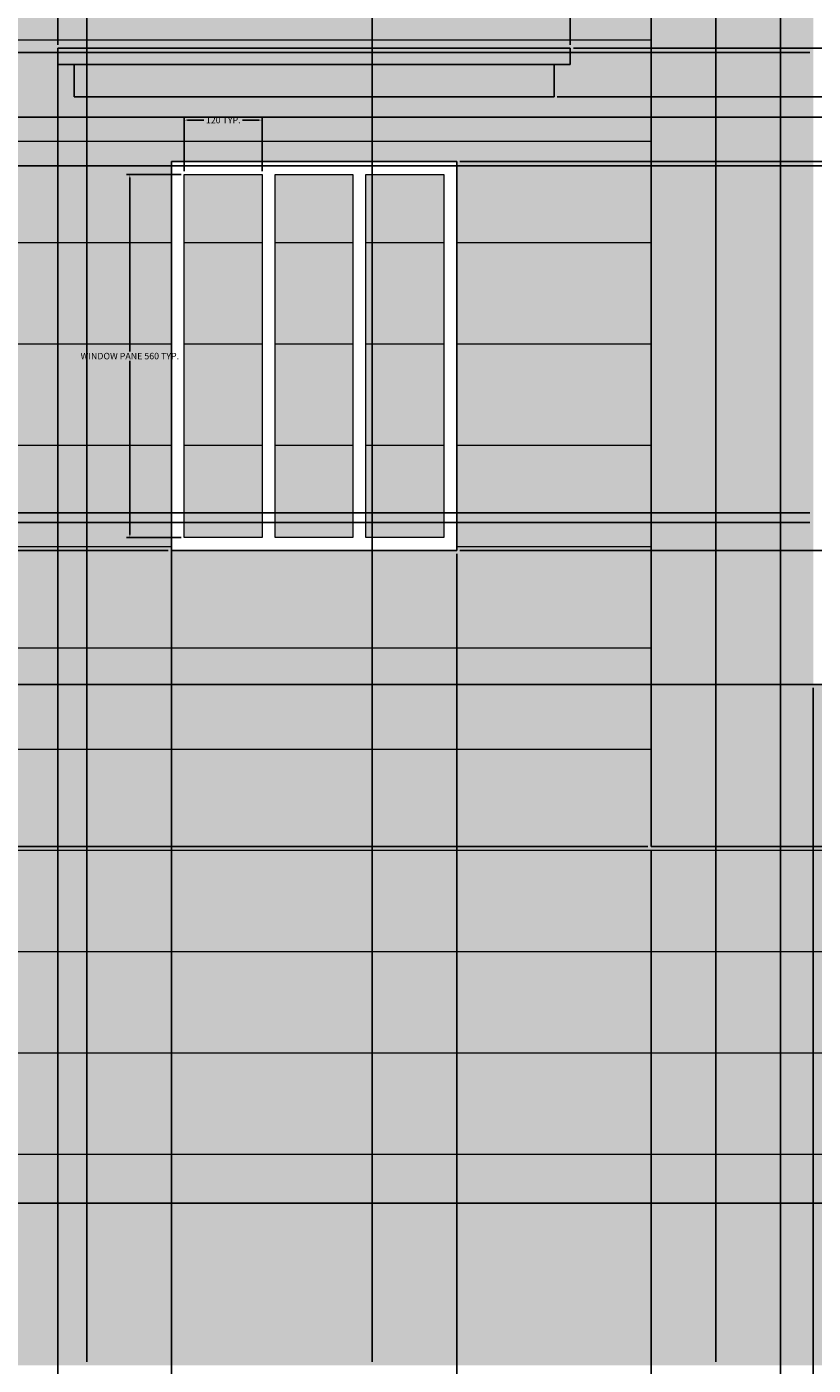
# Model space of a CAD drawing. Units: millimetres. Extents: x 2970 to 7764, y 2196 to 7505.
# Tile 9 of 13: x 4793 to 6006, y 4206 to 6270. Entities that reach past the tile are written whole.
import ezdxf

# ---------------------------------------------------------------- set-up
doc = ezdxf.new("R2010")
doc.units = ezdxf.units.MM
doc.header["$MEASUREMENT"] = 0
for name, color, linetype, lineweight in [('A-ANNO-DIMS', 2, 'Continuous', 18), ('A-ELEV', 7, 'Continuous', 25), ('A-ELEV-PATT', 8, 'Continuous', 13), ('A-GLAZ', 4, 'Continuous', 18)]:
    doc.layers.add(name, color=color, linetype=linetype, lineweight=lineweight)
doc.styles.get("Standard").update_dxf_attribs({"font": 'arial.ttf'})
doc.dimstyles.get("Standard").update_dxf_attribs({"dimtxt": 10, "dimasz": 5, "dimexe": 5, "dimexo": 5, "dimgap": 2, "dimtad": 0, "dimtih": 1, "dimtoh": 1, "dimdec": 0, "dimzin": 0, "dimdsep": 46, "dimtxsty": 'Standard', "dimcen": 2, "dimadec": 0, "dimazin": 0, "dimtfac": 1, "dimtdec": 0, "dimtofl": 0, "dimtmove": 0, "dimatfit": 3, "dimfxl": 1, "dimtolj": 1, "dimtzin": 0, "dimarcsym": 0})

# ---------------------------------------------------------------- blocks, each defined once
blk = doc.blocks.new('WIN-PANE')
blk.add_line((120, 560), (120, 0))
blk.add_lwpolyline([(120, 0), (0, 0), (0, 560), (120, 560)])
blk = doc.blocks.new('*D4')
at = {"layer": 'A-ANNO-DIMS', "color": 0, "lineweight": -2, "transparency": 16777216}
for p, q in [((5030.8, 6042.5), (4946.8, 6042.5)), ((4951.8, 6037.5), (4951.8, 5769.7)), ((4951.8, 5487.5), (4951.8, 5755.3)), ((5030.8, 5482.5), (4946.8, 5482.5))]:
    blk.add_line(p, q, dxfattribs=at)
at = {"layer": 'A-ANNO-DIMS', "color": 0, "transparency": 16777216}
for points in [[(4951, 6037.5), (4952.6, 6037.5), (4951.8, 6042.5)], [(4951, 5487.5), (4952.6, 5487.5), (4951.8, 5482.5)]]:
    blk.add_solid(points, dxfattribs=at)
at = {"layer": 'Defpoints', "color": 0, "transparency": 16777216}
for p in [(4951.8, 6042.5), (5035.8, 6042.5), (5035.8, 5482.5)]:
    blk.add_point(p, dxfattribs=at)
at = {"layer": 'A-ANNO-DIMS', "color": 0, "transparency": 16777216, "insert": (4951.8, 5762.5), "char_height": 10, "attachment_point": 5}
blk.add_mtext('\\A1;WINDOW PANE 560 TYP.', dxfattribs=at)
blk = doc.blocks.new('*D5')
at = {"layer": 'A-ANNO-DIMS', "color": 0, "lineweight": -2, "transparency": 16777216}
for p, q in [((5035.8, 6047.5), (5035.8, 6131.5)), ((5040.8, 6126.5), (5066.1, 6126.5)), ((5150.8, 6126.5), (5125.6, 6126.5)), ((5155.8, 6047.5), (5155.8, 6131.5))]:
    blk.add_line(p, q, dxfattribs=at)
at = {"layer": 'A-ANNO-DIMS', "color": 0, "transparency": 16777216}
for points in [[(5040.8, 6127.3), (5040.8, 6125.7), (5035.8, 6126.5)], [(5150.8, 6127.3), (5150.8, 6125.7), (5155.8, 6126.5)]]:
    blk.add_solid(points, dxfattribs=at)
at = {"layer": 'Defpoints', "color": 0, "transparency": 16777216}
for p in [(5155.8, 6126.5), (5035.8, 6042.5), (5155.8, 6042.5)]:
    blk.add_point(p, dxfattribs=at)
at = {"layer": 'A-ANNO-DIMS', "color": 0, "transparency": 16777216, "insert": (5095.8, 6126.5), "char_height": 10, "attachment_point": 5}
blk.add_mtext('\\A1;120 TYP.', dxfattribs=at)
blk = doc.blocks.new('*D34')
at = {"layer": 'A-ANNO-DIMS', "color": 0, "lineweight": -2, "transparency": 16777216}
for p, q in [((4355.5, 4210.8), (4355.5, 7503.8)), ((4360.5, 7498.8), (4607.5, 7498.8)), ((4880.5, 7498.8), (4633.5, 7498.8)), ((4885.5, 4210.8), (4885.5, 7503.8))]:
    blk.add_line(p, q, dxfattribs=at)
at = {"layer": 'A-ANNO-DIMS', "color": 0, "transparency": 16777216}
for points in [[(4360.5, 7499.6), (4360.5, 7498), (4355.5, 7498.8)], [(4880.5, 7499.6), (4880.5, 7498), (4885.5, 7498.8)]]:
    blk.add_solid(points, dxfattribs=at)
at = {"layer": 'Defpoints', "color": 0, "transparency": 16777216}
for p in [(4885.5, 7498.8), (4355.5, 4205.8), (4885.5, 4205.8)]:
    blk.add_point(p, dxfattribs=at)
at = {"layer": 'A-ANNO-DIMS', "color": 0, "transparency": 16777216, "insert": (4620.5, 7498.8), "char_height": 10, "attachment_point": 5}
blk.add_mtext('\\A1;530', dxfattribs=at)
blk = doc.blocks.new('*D35')
at = {"layer": 'A-ANNO-DIMS', "color": 0, "lineweight": -2, "transparency": 16777216}
for p, q in [((4885.5, 4210.8), (4885.5, 7503.8)), ((4890.5, 7498.8), (5092.3, 7498.8)), ((5320.5, 7498.8), (5118.7, 7498.8)), ((5325.5, 4210.8), (5325.5, 7503.8))]:
    blk.add_line(p, q, dxfattribs=at)
at = {"layer": 'A-ANNO-DIMS', "color": 0, "transparency": 16777216}
for points in [[(4890.5, 7499.6), (4890.5, 7498), (4885.5, 7498.8)], [(5320.5, 7499.6), (5320.5, 7498), (5325.5, 7498.8)]]:
    blk.add_solid(points, dxfattribs=at)
at = {"layer": 'Defpoints', "color": 0, "transparency": 16777216}
for p in [(5325.5, 7498.8), (4885.5, 4205.8), (5325.5, 4205.8)]:
    blk.add_point(p, dxfattribs=at)
at = {"layer": 'A-ANNO-DIMS', "color": 0, "transparency": 16777216, "insert": (5105.5, 7498.8), "char_height": 10, "attachment_point": 5}
blk.add_mtext('\\A1;440', dxfattribs=at)
blk = doc.blocks.new('*D36')
at = {"layer": 'A-ANNO-DIMS', "color": 0, "lineweight": -2, "transparency": 16777216}
for p, q in [((5325.5, 4210.8), (5325.5, 7503.8)), ((5330.5, 7498.8), (5571.5, 7498.8)), ((5850.3, 7498.8), (5609.3, 7498.8)), ((5855.3, 4210.8), (5855.3, 7503.8))]:
    blk.add_line(p, q, dxfattribs=at)
at = {"layer": 'A-ANNO-DIMS', "color": 0, "transparency": 16777216}
for points in [[(5330.5, 7499.6), (5330.5, 7498), (5325.5, 7498.8)], [(5850.3, 7499.6), (5850.3, 7498), (5855.3, 7498.8)]]:
    blk.add_solid(points, dxfattribs=at)
at = {"layer": 'Defpoints', "color": 0, "transparency": 16777216}
for p in [(5855.3, 7498.8), (5325.5, 4205.8), (5855.3, 4205.8)]:
    blk.add_point(p, dxfattribs=at)
at = {"layer": 'A-ANNO-DIMS', "color": 0, "transparency": 16777216, "insert": (5590.4, 7498.8), "char_height": 10, "attachment_point": 5}
blk.add_mtext('\\A1;529.8', dxfattribs=at)
blk = doc.blocks.new('*D37')
at = {"layer": 'A-ANNO-DIMS', "color": 0, "lineweight": -2, "transparency": 16777216}
for p, q in [((5855.3, 4210.8), (5855.3, 7503.8)), ((5860.3, 7498.8), (5892.7, 7498.8)), ((5950.3, 7498.8), (5917.8, 7498.8)), ((5955.3, 4010.8), (5955.3, 7503.8))]:
    blk.add_line(p, q, dxfattribs=at)
at = {"layer": 'A-ANNO-DIMS', "color": 0, "transparency": 16777216}
for points in [[(5860.3, 7499.6), (5860.3, 7498), (5855.3, 7498.8)], [(5950.3, 7499.6), (5950.3, 7498), (5955.3, 7498.8)]]:
    blk.add_solid(points, dxfattribs=at)
at = {"layer": 'Defpoints', "color": 0, "transparency": 16777216}
for p in [(5955.3, 7498.8), (5855.3, 4205.8), (5955.3, 4005.8)]:
    blk.add_point(p, dxfattribs=at)
at = {"layer": 'A-ANNO-DIMS', "color": 0, "transparency": 16777216, "insert": (5905.3, 7498.8), "char_height": 10, "attachment_point": 5}
blk.add_mtext('\\A1;100', dxfattribs=at)
blk = doc.blocks.new('*D39')
at = {"layer": 'A-ANNO-DIMS', "color": 0, "lineweight": -2, "transparency": 16777216}
for p, q in [((5955.3, 4010.8), (5955.3, 7503.8)), ((5960.3, 7498.8), (6117.2, 7498.8)), ((6300.3, 7498.8), (6143.3, 7498.8)), ((6305.3, 4010.8), (6305.3, 7503.8))]:
    blk.add_line(p, q, dxfattribs=at)
at = {"layer": 'A-ANNO-DIMS', "color": 0, "transparency": 16777216}
for points in [[(5960.3, 7499.6), (5960.3, 7498), (5955.3, 7498.8)], [(6300.3, 7499.6), (6300.3, 7498), (6305.3, 7498.8)]]:
    blk.add_solid(points, dxfattribs=at)
at = {"layer": 'Defpoints', "color": 0, "transparency": 16777216}
for p in [(6305.3, 7498.8), (5955.3, 4005.8), (6305.3, 4005.8)]:
    blk.add_point(p, dxfattribs=at)
at = {"layer": 'A-ANNO-DIMS', "color": 0, "transparency": 16777216, "insert": (6130.3, 7498.8), "char_height": 10, "attachment_point": 5}
blk.add_mtext('\\A1;350', dxfattribs=at)
blk = doc.blocks.new('*D46')
at = {"layer": 'A-ANNO-DIMS', "color": 0, "lineweight": -2, "transparency": 16777216}
for p, q in [((4350.5, 4205.8), (2982.5, 4205.8)), ((2987.5, 4200.8), (2987.5, 3912.9)), ((2987.5, 3610.8), (2987.5, 3898.7)), ((4880.5, 3605.8), (2982.5, 3605.8))]:
    blk.add_line(p, q, dxfattribs=at)
at = {"layer": 'A-ANNO-DIMS', "color": 0, "transparency": 16777216}
for points in [[(2986.7, 4200.8), (2988.3, 4200.8), (2987.5, 4205.8)], [(2986.7, 3610.8), (2988.3, 3610.8), (2987.5, 3605.8)]]:
    blk.add_solid(points, dxfattribs=at)
at = {"layer": 'Defpoints', "color": 0, "transparency": 16777216}
for p in [(2987.5, 4205.8), (4355.5, 4205.8), (4885.5, 3605.8)]:
    blk.add_point(p, dxfattribs=at)
at = {"layer": 'A-ANNO-DIMS', "color": 0, "transparency": 16777216, "insert": (2987.5, 3905.8), "char_height": 10, "attachment_point": 5}
blk.add_mtext('\\A1;600', dxfattribs=at)
blk = doc.blocks.new('*D56')
at = {"layer": 'A-ANNO-DIMS', "color": 0, "lineweight": -2, "transparency": 16777216}
for p, q in [((5015.8, 5457.5), (5015.8, 2197.8)), ((5455.8, 5457.5), (5455.8, 2197.8)), ((5020.8, 2202.8), (5222.6, 2202.8)), ((5450.8, 2202.8), (5249, 2202.8))]:
    blk.add_line(p, q, dxfattribs=at)
at = {"layer": 'A-ANNO-DIMS', "color": 0, "transparency": 16777216}
for points in [[(5020.8, 2203.6), (5020.8, 2202), (5015.8, 2202.8)], [(5450.8, 2203.6), (5450.8, 2202), (5455.8, 2202.8)]]:
    blk.add_solid(points, dxfattribs=at)
at = {"layer": 'Defpoints', "color": 0, "transparency": 16777216}
for p in [(5015.8, 5462.5), (5455.8, 5462.5), (5455.8, 2202.8)]:
    blk.add_point(p, dxfattribs=at)
at = {"layer": 'A-ANNO-DIMS', "color": 0, "transparency": 16777216, "insert": (5235.8, 2202.8), "char_height": 10, "attachment_point": 5}
blk.add_mtext('\\A1;440', dxfattribs=at)
blk = doc.blocks.new('*D57')
at = {"layer": 'A-ANNO-DIMS', "color": 0, "lineweight": -2, "transparency": 16777216}
for p, q in [((5455.8, 5457.5), (5455.8, 2197.8)), ((5755.5, 5000.8), (5755.5, 2197.8)), ((5460.8, 2202.8), (5586.7, 2202.8)), ((5750.5, 2202.8), (5624.6, 2202.8))]:
    blk.add_line(p, q, dxfattribs=at)
at = {"layer": 'A-ANNO-DIMS', "color": 0, "transparency": 16777216}
for points in [[(5460.8, 2203.6), (5460.8, 2202), (5455.8, 2202.8)], [(5750.5, 2203.6), (5750.5, 2202), (5755.5, 2202.8)]]:
    blk.add_solid(points, dxfattribs=at)
at = {"layer": 'Defpoints', "color": 0, "transparency": 16777216}
for p in [(5455.8, 5462.5), (5755.5, 5005.8), (5755.5, 2202.8)]:
    blk.add_point(p, dxfattribs=at)
at = {"layer": 'A-ANNO-DIMS', "color": 0, "transparency": 16777216, "insert": (5605.7, 2202.8), "char_height": 10, "attachment_point": 5}
blk.add_mtext('\\A1;299.7', dxfattribs=at)
blk = doc.blocks.new('*D58')
at = {"layer": 'A-ANNO-DIMS', "color": 0, "lineweight": -2, "transparency": 16777216}
for p, q in [((6005.5, 5250.8), (6005.5, 2197.8)), ((5755.5, 5000.8), (5755.5, 2197.8)), ((5760.5, 2202.8), (5867.4, 2202.8)), ((6000.5, 2202.8), (5893.6, 2202.8))]:
    blk.add_line(p, q, dxfattribs=at)
at = {"layer": 'A-ANNO-DIMS', "color": 0, "transparency": 16777216}
for points in [[(5760.5, 2203.6), (5760.5, 2202), (5755.5, 2202.8)], [(6000.5, 2203.6), (6000.5, 2202), (6005.5, 2202.8)]]:
    blk.add_solid(points, dxfattribs=at)
at = {"layer": 'Defpoints', "color": 0, "transparency": 16777216}
for p in [(6005.5, 5255.8), (5755.5, 5005.8), (6005.5, 2202.8)]:
    blk.add_point(p, dxfattribs=at)
at = {"layer": 'A-ANNO-DIMS', "color": 0, "transparency": 16777216, "insert": (5880.5, 2202.8), "char_height": 10, "attachment_point": 5}
blk.add_mtext('\\A1;250', dxfattribs=at)
blk = doc.blocks.new('*D59')
at = {"layer": 'A-ANNO-DIMS', "color": 0, "lineweight": -2, "transparency": 16777216}
for p, q in [((6005.5, 5250.8), (6005.5, 2197.8)), ((7155.5, 5250.8), (7155.5, 2197.8)), ((6010.5, 2202.8), (6564.1, 2202.8)), ((7150.5, 2202.8), (6596.9, 2202.8))]:
    blk.add_line(p, q, dxfattribs=at)
at = {"layer": 'A-ANNO-DIMS', "color": 0, "transparency": 16777216}
for points in [[(6010.5, 2203.6), (6010.5, 2202), (6005.5, 2202.8)], [(7150.5, 2203.6), (7150.5, 2202), (7155.5, 2202.8)]]:
    blk.add_solid(points, dxfattribs=at)
at = {"layer": 'Defpoints', "color": 0, "transparency": 16777216}
for p in [(6005.5, 5255.8), (7155.5, 5255.8), (7155.5, 2202.8)]:
    blk.add_point(p, dxfattribs=at)
at = {"layer": 'A-ANNO-DIMS', "color": 0, "transparency": 16777216, "insert": (6580.5, 2202.8), "char_height": 10, "attachment_point": 5}
blk.add_mtext('\\A1;1150', dxfattribs=at)
blk = doc.blocks.new('*D61')
at = {"layer": 'A-ANNO-DIMS', "color": 0, "lineweight": -2, "transparency": 16777216}
for p, q in [((5010.8, 5462.5), (2982.5, 5462.5)), ((2987.5, 5457.5), (2987.5, 5241.2)), ((2987.5, 5010.8), (2987.5, 5227)), ((5750.5, 5005.8), (2982.5, 5005.8))]:
    blk.add_line(p, q, dxfattribs=at)
at = {"layer": 'A-ANNO-DIMS', "color": 0, "transparency": 16777216}
for points in [[(2986.7, 5457.5), (2988.3, 5457.5), (2987.5, 5462.5)], [(2986.7, 5010.8), (2988.3, 5010.8), (2987.5, 5005.8)]]:
    blk.add_solid(points, dxfattribs=at)
at = {"layer": 'Defpoints', "color": 0, "transparency": 16777216}
for p in [(5015.8, 5462.5), (2987.5, 5005.8), (5755.5, 5005.8)]:
    blk.add_point(p, dxfattribs=at)
at = {"layer": 'A-ANNO-DIMS', "color": 0, "transparency": 16777216, "insert": (2987.5, 5234.1), "char_height": 10, "attachment_point": 5}
blk.add_mtext('\\A1;456.7', dxfattribs=at)
blk = doc.blocks.new('*D62')
at = {"layer": 'A-ANNO-DIMS', "color": 0, "lineweight": -2, "transparency": 16777216}
for p, q in [((5460.8, 6062.5), (7753.5, 6062.5)), ((7748.5, 6057.5), (7748.5, 5769.6)), ((7748.5, 5467.5), (7748.5, 5755.4)), ((5460.8, 5462.5), (7753.5, 5462.5))]:
    blk.add_line(p, q, dxfattribs=at)
at = {"layer": 'A-ANNO-DIMS', "color": 0, "transparency": 16777216}
for points in [[(7747.7, 6057.5), (7749.3, 6057.5), (7748.5, 6062.5)], [(7747.7, 5467.5), (7749.3, 5467.5), (7748.5, 5462.5)]]:
    blk.add_solid(points, dxfattribs=at)
at = {"layer": 'Defpoints', "color": 0, "transparency": 16777216}
for p in [(5455.8, 6062.5), (7748.5, 6062.5), (5455.8, 5462.5)]:
    blk.add_point(p, dxfattribs=at)
at = {"layer": 'A-ANNO-DIMS', "color": 0, "transparency": 16777216, "insert": (7748.5, 5762.5), "char_height": 10, "attachment_point": 5}
blk.add_mtext('\\A1;600', dxfattribs=at)
blk = doc.blocks.new('*D63')
at = {"layer": 'A-ANNO-DIMS', "color": 0, "lineweight": -2, "transparency": 16777216}
for p, q in [((5610.8, 6162.5), (7753.5, 6162.5)), ((7748.5, 6157.5), (7748.5, 6119.6)), ((7748.5, 6067.5), (7748.5, 6105.4)), ((5460.8, 6062.5), (7753.5, 6062.5))]:
    blk.add_line(p, q, dxfattribs=at)
at = {"layer": 'A-ANNO-DIMS', "color": 0, "transparency": 16777216}
for points in [[(7747.7, 6157.5), (7749.3, 6157.5), (7748.5, 6162.5)], [(7747.7, 6067.5), (7749.3, 6067.5), (7748.5, 6062.5)]]:
    blk.add_solid(points, dxfattribs=at)
at = {"layer": 'Defpoints', "color": 0, "transparency": 16777216}
for p in [(5605.8, 6162.5), (7748.5, 6162.5), (5455.8, 6062.5)]:
    blk.add_point(p, dxfattribs=at)
at = {"layer": 'A-ANNO-DIMS', "color": 0, "transparency": 16777216, "insert": (7748.5, 6112.5), "char_height": 10, "attachment_point": 5}
blk.add_mtext('\\A1;100', dxfattribs=at)
blk = doc.blocks.new('*D64')
at = {"layer": 'A-ANNO-DIMS', "color": 0, "lineweight": -2, "transparency": 16777216}
for p, q in [((5635.8, 6237.5), (7753.5, 6237.5)), ((7748.5, 6232.5), (7748.5, 6207.1)), ((7748.5, 6167.5), (7748.5, 6192.9)), ((5610.8, 6162.5), (7753.5, 6162.5))]:
    blk.add_line(p, q, dxfattribs=at)
at = {"layer": 'A-ANNO-DIMS', "color": 0, "transparency": 16777216}
for points in [[(7747.7, 6232.5), (7749.3, 6232.5), (7748.5, 6237.5)], [(7747.7, 6167.5), (7749.3, 6167.5), (7748.5, 6162.5)]]:
    blk.add_solid(points, dxfattribs=at)
at = {"layer": 'Defpoints', "color": 0, "transparency": 16777216}
for p in [(5630.8, 6237.5), (7748.5, 6237.5), (5605.8, 6162.5)]:
    blk.add_point(p, dxfattribs=at)
at = {"layer": 'A-ANNO-DIMS', "color": 0, "transparency": 16777216, "insert": (7748.5, 6200), "char_height": 10, "attachment_point": 5}
blk.add_mtext('\\A1;75', dxfattribs=at)
blk = doc.blocks.new('*D65')
at = {"layer": 'A-ANNO-DIMS', "color": 0, "lineweight": -2, "transparency": 16777216}
for p, q in [((4840.8, 6242.5), (4840.8, 7503.8)), ((4845.8, 7498.8), (5222.8, 7498.8)), ((5625.8, 7498.8), (5248.8, 7498.8)), ((5630.8, 6242.5), (5630.8, 7503.8))]:
    blk.add_line(p, q, dxfattribs=at)
at = {"layer": 'A-ANNO-DIMS', "color": 0, "transparency": 16777216}
for points in [[(4845.8, 7499.6), (4845.8, 7498), (4840.8, 7498.8)], [(5625.8, 7499.6), (5625.8, 7498), (5630.8, 7498.8)]]:
    blk.add_solid(points, dxfattribs=at)
at = {"layer": 'Defpoints', "color": 0, "transparency": 16777216}
for p in [(5630.8, 7498.8), (4840.8, 6237.5), (5630.8, 6237.5)]:
    blk.add_point(p, dxfattribs=at)
at = {"layer": 'A-ANNO-DIMS', "color": 0, "transparency": 16777216, "insert": (5235.8, 7498.8), "char_height": 10, "attachment_point": 5}
blk.add_mtext('\\A1;790', dxfattribs=at)
blk = doc.blocks.new('*D66')
at = {"layer": 'A-ANNO-DIMS', "color": 0, "lineweight": -2, "transparency": 16777216}
for p, q in [((4840.8, 6232.5), (4840.8, 2197.8)), ((5015.8, 6057.5), (5015.8, 2197.8)), ((4845.8, 2202.8), (4915.7, 2202.8)), ((5010.8, 2202.8), (4940.9, 2202.8))]:
    blk.add_line(p, q, dxfattribs=at)
at = {"layer": 'A-ANNO-DIMS', "color": 0, "transparency": 16777216}
for points in [[(4845.8, 2203.6), (4845.8, 2202), (4840.8, 2202.8)], [(5010.8, 2203.6), (5010.8, 2202), (5015.8, 2202.8)]]:
    blk.add_solid(points, dxfattribs=at)
at = {"layer": 'Defpoints', "color": 0, "transparency": 16777216}
for p in [(4840.8, 6237.5), (5015.8, 6062.5), (5015.8, 2202.8)]:
    blk.add_point(p, dxfattribs=at)
at = {"layer": 'A-ANNO-DIMS', "color": 0, "transparency": 16777216, "insert": (4928.3, 2202.8), "char_height": 10, "attachment_point": 5}
blk.add_mtext('\\A1;175', dxfattribs=at)
blk = doc.blocks.new('*D76')
at = {"layer": 'A-ANNO-DIMS', "color": 0, "lineweight": -2, "transparency": 16777216}
for p, q in [((6100.5, 6055.8), (2982.5, 6055.8)), ((2987.5, 6050.8), (2987.5, 5662.9)), ((2987.5, 5260.8), (2987.5, 5648.7)), ((6100.5, 5255.8), (2982.5, 5255.8))]:
    blk.add_line(p, q, dxfattribs=at)
at = {"layer": 'A-ANNO-DIMS', "color": 0, "transparency": 16777216}
for points in [[(2986.7, 6050.8), (2988.3, 6050.8), (2987.5, 6055.8)], [(2986.7, 5260.8), (2988.3, 5260.8), (2987.5, 5255.8)]]:
    blk.add_solid(points, dxfattribs=at)
at = {"layer": 'Defpoints', "color": 0, "transparency": 16777216}
for p in [(2987.5, 6055.8), (6105.5, 6055.8), (6105.5, 5255.8)]:
    blk.add_point(p, dxfattribs=at)
at = {"layer": 'A-ANNO-DIMS', "color": 0, "transparency": 16777216, "insert": (2987.5, 5655.8), "char_height": 10, "attachment_point": 5}
blk.add_mtext('\\A1;800', dxfattribs=at)
blk = doc.blocks.new('*D77')
at = {"layer": 'A-ANNO-DIMS', "color": 0, "lineweight": -2, "transparency": 16777216}
for p, q in [((6960.5, 5405.8), (7753.5, 5405.8)), ((7748.5, 5400.8), (7748.5, 5337.9)), ((7748.5, 5260.8), (7748.5, 5323.7)), ((6010.5, 5255.8), (7753.5, 5255.8))]:
    blk.add_line(p, q, dxfattribs=at)
at = {"layer": 'A-ANNO-DIMS', "color": 0, "transparency": 16777216}
for points in [[(7747.7, 5400.8), (7749.3, 5400.8), (7748.5, 5405.8)], [(7747.7, 5260.8), (7749.3, 5260.8), (7748.5, 5255.8)]]:
    blk.add_solid(points, dxfattribs=at)
at = {"layer": 'Defpoints', "color": 0, "transparency": 16777216}
for p in [(6955.5, 5405.8), (7748.5, 5405.8), (6005.5, 5255.8)]:
    blk.add_point(p, dxfattribs=at)
at = {"layer": 'A-ANNO-DIMS', "color": 0, "transparency": 16777216, "insert": (7748.5, 5330.8), "char_height": 10, "attachment_point": 5}
blk.add_mtext('\\A1;150', dxfattribs=at)
blk = doc.blocks.new('*D79')
at = {"layer": 'A-ANNO-DIMS', "color": 0, "lineweight": -2, "transparency": 16777216}
for p, q in [((6000.5, 5505.8), (2982.5, 5505.8)), ((2987.5, 5500.8), (2987.5, 5387.9)), ((2987.5, 5260.8), (2987.5, 5373.7)), ((6000.5, 5255.8), (2982.5, 5255.8))]:
    blk.add_line(p, q, dxfattribs=at)
at = {"layer": 'A-ANNO-DIMS', "color": 0, "transparency": 16777216}
for points in [[(2986.7, 5500.8), (2988.3, 5500.8), (2987.5, 5505.8)], [(2986.7, 5260.8), (2988.3, 5260.8), (2987.5, 5255.8)]]:
    blk.add_solid(points, dxfattribs=at)
at = {"layer": 'Defpoints', "color": 0, "transparency": 16777216}
for p in [(2987.5, 5505.8), (6005.5, 5505.8), (6005.5, 5255.8)]:
    blk.add_point(p, dxfattribs=at)
at = {"layer": 'A-ANNO-DIMS', "color": 0, "transparency": 16777216, "insert": (2987.5, 5380.8), "char_height": 10, "attachment_point": 5}
blk.add_mtext('\\A1;250', dxfattribs=at)
blk = doc.blocks.new('*D80')
at = {"layer": 'A-ANNO-DIMS', "color": 0, "lineweight": -2, "transparency": 16777216}
for p, q in [((6000.5, 5520.8), (2982.5, 5520.8)), ((2987.5, 5525.8), (2987.5, 5530.8)), ((6000.5, 5505.8), (2982.5, 5505.8)), ((2987.5, 5500.8), (2987.5, 5495.8))]:
    blk.add_line(p, q, dxfattribs=at)
at = {"layer": 'A-ANNO-DIMS', "color": 0, "transparency": 16777216}
for points in [[(2986.7, 5525.8), (2988.3, 5525.8), (2987.5, 5520.8)], [(2986.7, 5500.8), (2988.3, 5500.8), (2987.5, 5505.8)]]:
    blk.add_solid(points, dxfattribs=at)
at = {"layer": 'Defpoints', "color": 0, "transparency": 16777216}
for p in [(2987.5, 5520.8), (6005.5, 5520.8), (6005.5, 5505.8)]:
    blk.add_point(p, dxfattribs=at)
at = {"layer": 'A-ANNO-DIMS', "color": 0, "transparency": 16777216, "insert": (2987.5, 5513.3), "char_height": 10, "attachment_point": 5}
blk.add_mtext('\\A1;15', dxfattribs=at)
blk = doc.blocks.new('*D81')
at = {"layer": 'A-ANNO-DIMS', "color": 0, "lineweight": -2, "transparency": 16777216}
for p, q in [((6000.5, 6230.8), (2982.5, 6230.8)), ((2987.5, 6225.8), (2987.5, 6187.9)), ((2987.5, 6135.8), (2987.5, 6173.7)), ((6025.5, 6130.8), (2982.5, 6130.8))]:
    blk.add_line(p, q, dxfattribs=at)
at = {"layer": 'A-ANNO-DIMS', "color": 0, "transparency": 16777216}
for points in [[(2986.7, 6225.8), (2988.3, 6225.8), (2987.5, 6230.8)], [(2986.7, 6135.8), (2988.3, 6135.8), (2987.5, 6130.8)]]:
    blk.add_solid(points, dxfattribs=at)
at = {"layer": 'Defpoints', "color": 0, "transparency": 16777216}
for p in [(2987.5, 6230.8), (6005.5, 6230.8), (6030.5, 6130.8)]:
    blk.add_point(p, dxfattribs=at)
at = {"layer": 'A-ANNO-DIMS', "color": 0, "transparency": 16777216, "insert": (2987.5, 6180.8), "char_height": 10, "attachment_point": 5}
blk.add_mtext('\\A1;100', dxfattribs=at)
blk = doc.blocks.new('*D82')
at = {"layer": 'A-ANNO-DIMS', "color": 0, "lineweight": -2, "transparency": 16777216}
for p, q in [((6000.5, 6505.8), (2982.5, 6505.8)), ((2987.5, 6500.8), (2987.5, 6375.4)), ((2987.5, 6235.8), (2987.5, 6361.2)), ((6000.5, 6230.8), (2982.5, 6230.8))]:
    blk.add_line(p, q, dxfattribs=at)
at = {"layer": 'A-ANNO-DIMS', "color": 0, "transparency": 16777216}
for points in [[(2986.7, 6500.8), (2988.3, 6500.8), (2987.5, 6505.8)], [(2986.7, 6235.8), (2988.3, 6235.8), (2987.5, 6230.8)]]:
    blk.add_solid(points, dxfattribs=at)
at = {"layer": 'Defpoints', "color": 0, "transparency": 16777216}
for p in [(2987.5, 6505.8), (6005.5, 6505.8), (6005.5, 6230.8)]:
    blk.add_point(p, dxfattribs=at)
at = {"layer": 'A-ANNO-DIMS', "color": 0, "transparency": 16777216, "insert": (2987.5, 6368.3), "char_height": 10, "attachment_point": 5}
blk.add_mtext('\\A1;275', dxfattribs=at)

msp = doc.modelspace()

# ---------------------------------------------------------------- hatches: boundary and pattern name
at = {"layer": 'A-ELEV-PATT'}
h = msp.add_hatch(color=256, dxfattribs=at)
h.dxf.hatch_style = 1
h.paths.add_polyline_path([(6405.5, 7255.789), (4305.5, 7255.789), (4305.5, 6505.789), (3730.5, 6505.789), (3730.5, 4205.789), (3730.5, 2945.789), (3730.5, 2895.789), (3830.5, 2895.789), (3830.5, 4205.789), (3830.5, 6405.789), (4405.5, 6405.789), (4405.5, 4205.789), (6905.5, 4205.789), (6905.5, 2945.789), (6905.5, 2845.789), (7155.5, 2845.789), (7155.5, 2945.789), (7155.5, 4205.789), (7155.5, 4455.789), (4555.5, 4455.789), (4555.5, 6505.789), (4555.5, 7005.789), (6155.5, 7005.789), (6155.5, 6755.789), (6405.5, 6755.789)])
h.paths.add_polyline_path([(7405.5, 6755.789), (6155.5, 6755.789), (5755.5, 6755.789), (5755.5, 5005.789), (7405.5, 5005.789)])
h.paths.add_polyline_path([(7155.5, 6505.789), (7155.5, 5255.789), (6005.5, 5255.789), (6005.5, 6505.789)], flags=16)
h.paths.add_polyline_path([(6105.5, 5520.789), (6105.5, 6055.789), (6455.5, 6055.789), (6455.5, 5520.789), (6655.5, 5520.789), (6655.5, 5605.789), (6655.5, 5955.789), (6955.5, 5955.789), (6955.5, 5605.789), (6955.5, 5520.789)], flags=0)
h.paths.add_polyline_path([(6425.5, 5755.789), (6425.5, 5655.789), (6425.5, 5555.789), (6405.5, 5555.789), (6405.5, 5755.789)], flags=0)
h.paths.add_polyline_path([(6955.5, 5505.789), (6955.5, 5405.789), (6655.5, 5405.789), (6655.5, 5505.789)], flags=0)
h = msp.add_hatch(color=256, dxfattribs=at)
h.set_gradient(color1=(147, 149, 152), color2=(199, 200, 202), name='CURVED')
h.paths.add_polyline_path([(6955.5, 4455.789), (6955.5, 5005.789), (5755.5, 5005.789), (5755.5, 6755.789), (6155.5, 6755.789), (6155.5, 7005.789), (4555.5, 7005.789), (4555.5, 6505.789), (4555.5, 4455.789)])
h.paths.add_polyline_path([(5015.81, 5462.49), (5015.81, 6062.49), (5455.81, 6062.49), (5455.81, 5462.49)], flags=16)
h.paths.add_polyline_path([(5035.81, 5482.49), (5035.81, 6042.49), (5155.81, 6042.49), (5155.81, 5482.49)], flags=0)
h.paths.add_polyline_path([(5175.81, 5482.49), (5175.81, 6042.49), (5295.81, 6042.49), (5295.81, 5482.49)], flags=0)
h.paths.add_polyline_path([(5315.81, 5482.49), (5315.81, 6042.49), (5435.81, 6042.49), (5435.81, 5482.49)], flags=0)
h.paths.add_polyline_path([(4865.81, 6162.49), (4865.81, 6212.49), (4840.81, 6212.49), (4840.81, 6237.49), (5630.81, 6237.49), (5630.81, 6212.49), (5605.81, 6212.49), (5605.81, 6162.49), (5015.81, 6162.49)], flags=16)
h = msp.add_hatch(dxfattribs=at)
h.set_pattern_fill('ANSI31', color=256, scale=1250, angle=135, style=0)
h.paths.add_polyline_path([(5755.5, 6755.789), (6155.5, 6755.789), (6155.5, 7005.789), (4555.5, 7005.789), (4555.5, 6505.789), (4555.5, 4455.789), (6955.5, 4455.789), (6955.5, 5005.789), (5755.5, 5005.789)])
h.paths.add_polyline_path([(5015.81, 5462.49), (5015.81, 6062.49), (5455.81, 6062.49), (5455.81, 5462.49)], flags=16)
h.paths.add_polyline_path([(5035.81, 5482.49), (5035.81, 6042.49), (5155.81, 6042.49), (5155.81, 5482.49)], flags=0)
h.paths.add_polyline_path([(5175.81, 5482.49), (5175.81, 6042.49), (5295.81, 6042.49), (5295.81, 5482.49)], flags=0)
h.paths.add_polyline_path([(5315.81, 5482.49), (5315.81, 6042.49), (5435.81, 6042.49), (5435.81, 5482.49)], flags=0)
h.paths.add_polyline_path([(4865.81, 6162.49), (4865.81, 6212.49), (4840.81, 6212.49), (4840.81, 6237.49), (5630.81, 6237.49), (5630.81, 6212.49), (5605.81, 6212.49), (5605.81, 6162.49), (5015.81, 6162.49)], flags=16)
h = msp.add_hatch(color=256, dxfattribs=at)
h.set_gradient(color1=(99, 100, 102), color2=(99, 100, 102), name='INVSPHERICAL')
h.paths.add_polyline_path([(4840.81, 6237.49), (4840.81, 6212.49), (4865.81, 6212.49), (5605.81, 6212.49), (5630.81, 6212.49), (5630.81, 6237.49)])
h = msp.add_hatch(color=256, dxfattribs=at)
h.set_gradient(color1=(255, 255, 255), color2=(199, 200, 202), name='INVSPHERICAL')
h.paths.add_polyline_path([(5605.81, 6162.49), (5605.81, 6212.49), (4865.81, 6212.49), (4865.81, 6162.49), (5015.81, 6162.49)])
h = msp.add_hatch(color=256, dxfattribs=at)
h.set_gradient(color1=(122, 175, 223), color2=(173, 221, 247), name='SPHERICAL')
h.paths.add_polyline_path([(5035.81, 5482.49), (5155.81, 5482.49), (5155.81, 6042.49), (5035.81, 6042.49)])
h.paths.add_polyline_path([(5295.81, 6042.49), (5175.81, 6042.49), (5175.81, 5482.49), (5295.81, 5482.49)])
h.paths.add_polyline_path([(5435.81, 6042.49), (5315.81, 6042.49), (5315.81, 5482.49), (5435.81, 5482.49)])

# ---------------------------------------------------------------- linework, layer by layer
at = {"layer": 'A-ELEV'}
for p, q in [((5755.5, 5005.789), (5755.5, 6755.789)), ((4840.81, 6212.49), (4840.81, 6237.49)), ((4840.81, 6237.49), (5630.81, 6237.49)), ((5630.81, 6212.49), (5630.81, 6237.49)), ((4865.81, 6212.49), (4840.81, 6212.49)), ((4865.81, 6162.49), (4865.81, 6212.49)), ((4865.81, 6212.49), (5605.81, 6212.49)), ((5605.81, 6162.49), (5605.81, 6212.49)), ((5605.81, 6212.49), (5630.81, 6212.49)), ((5015.81, 6162.49), (4865.81, 6162.49)), ((5015.81, 6162.49), (5605.81, 6162.49)), ((5015.81, 6062.49), (5455.81, 6062.49)), ((5015.81, 5462.49), (5015.81, 6062.49)), ((5455.81, 6062.49), (5455.81, 5462.49)), ((5455.81, 5462.49), (5015.81, 5462.49)), ((7405.5, 5005.789), (5755.5, 5005.789)), ((4555.5, 4455.789), (7155.5, 4455.789))]:
    msp.add_line(p, q, dxfattribs=at)

# ---------------------------------------------------------------- block references
at = {"layer": 'A-GLAZ'}
msp.add_blockref('WIN-PANE', (5035.81, 5482.49), dxfattribs=at)
at = {"layer": 'A-GLAZ', "rotation": 180}
for p in [(5295.81, 6042.49), (5435.81, 6042.49)]:
    msp.add_blockref('WIN-PANE', p, dxfattribs=at)

# ---------------------------------------------------------------- dimensions: what is measured, and where the dimension line sits
at = {"layer": 'A-ANNO-DIMS'}
for base, p1, p2, override, picture, middle in [((4885.5, 7498.789), (4355.5, 4205.789), (4885.5, 4205.789), {"dimdec": 0, "dimlfac": 1, "dimrnd": 0, "dimzin": 0, "dimdsep": 46, "dimlunit": 2}, '*D34', (4620.5, 7498.789)), ((5630.81, 7498.789), (4840.81, 6237.49), (5630.81, 6237.49), {"dimdec": 0, "dimlfac": 1, "dimrnd": 0, "dimzin": 0, "dimdsep": 46, "dimlunit": 2}, '*D65', (5235.81, 7498.789)), ((5325.5, 7498.789), (4885.5, 4205.789), (5325.5, 4205.789), {"dimdec": 0, "dimlfac": 1, "dimrnd": 0, "dimzin": 0, "dimdsep": 46, "dimlunit": 2}, '*D35', (5105.5, 7498.789)), ((5855.271, 7498.789), (5325.5, 4205.789), (5855.271, 4205.789), {"dimdec": 1, "dimlfac": 1, "dimrnd": 0, "dimzin": 0, "dimdsep": 46, "dimlunit": 2}, '*D36', (5590.386, 7498.789)), ((5955.271, 7498.789), (5855.271, 4205.789), (5955.271, 4005.789), {"dimdec": 0, "dimlfac": 1, "dimrnd": 0, "dimzin": 0, "dimdsep": 46, "dimlunit": 2}, '*D37', (5905.271, 7498.789)), ((6305.271, 7498.789), (5955.271, 4005.789), (6305.271, 4005.789), {"dimdec": 0, "dimlfac": 1, "dimrnd": 0, "dimzin": 0, "dimdsep": 46, "dimlunit": 2}, '*D39', (6130.271, 7498.789)), ((5015.81, 2202.789), (4840.81, 6237.49), (5015.81, 6062.49), {"dimdec": 0, "dimlfac": 1, "dimrnd": 0, "dimzin": 0, "dimdsep": 46, "dimlunit": 2}, '*D66', (4928.31, 2202.789)), ((5455.81, 2202.789), (5015.81, 5462.49), (5455.81, 5462.49), {"dimdec": 0, "dimlfac": 1, "dimrnd": 0, "dimzin": 0, "dimdsep": 46, "dimlunit": 2}, '*D56', (5235.81, 2202.789)), ((5755.5, 2202.789), (5455.81, 5462.49), (5755.5, 5005.789), {"dimdec": 1, "dimlfac": 1, "dimrnd": 0, "dimzin": 0, "dimdsep": 46, "dimlunit": 2}, '*D57', (5605.655, 2202.789)), ((6005.5, 2202.789), (5755.5, 5005.789), (6005.5, 5255.789), {"dimdec": 0, "dimlfac": 1, "dimrnd": 0, "dimzin": 0, "dimdsep": 46, "dimlunit": 2}, '*D58', (5880.5, 2202.789)), ((7155.5, 2202.789), (6005.5, 5255.789), (7155.5, 5255.789), {"dimdec": 0, "dimlfac": 1, "dimrnd": 0, "dimzin": 0, "dimdsep": 46, "dimlunit": 2}, '*D59', (6580.5, 2202.789))]:
    dim = msp.add_linear_dim(base=base, p1=p1, p2=p2, dimstyle='Standard', override=override, dxfattribs=at)
    dim.commit()
    dim.dimension.update_dxf_attribs({"geometry": picture, "text_midpoint": middle})
for base, p1, p2, override, picture, middle in [((2987.5, 6505.789), (6005.5, 6230.789), (6005.5, 6505.789), {"dimdec": 0, "dimlfac": 1, "dimrnd": 0, "dimzin": 0, "dimdsep": 46, "dimlunit": 2}, '*D82', (2987.5, 6368.289)), ((7748.5, 6237.49), (5605.81, 6162.49), (5630.81, 6237.49), {"dimdec": 0, "dimlfac": 1, "dimrnd": 0, "dimzin": 0, "dimdsep": 46, "dimlunit": 2}, '*D64', (7748.5, 6199.99)), ((2987.5, 6230.789), (6030.5, 6130.789), (6005.5, 6230.789), {"dimdec": 0, "dimlfac": 1, "dimrnd": 0, "dimzin": 0, "dimdsep": 46, "dimlunit": 2}, '*D81', (2987.5, 6180.789)), ((7748.5, 6162.49), (5455.81, 6062.49), (5605.81, 6162.49), {"dimdec": 0, "dimlfac": 1, "dimrnd": 0, "dimzin": 0, "dimdsep": 46, "dimlunit": 2}, '*D63', (7748.5, 6112.49)), ((2987.5, 6055.789), (6105.5, 5255.789), (6105.5, 6055.789), {"dimdec": 0, "dimlfac": 1, "dimrnd": 0, "dimzin": 0, "dimdsep": 46, "dimlunit": 2}, '*D76', (2987.5, 5655.789)), ((7748.5, 6062.49), (5455.81, 5462.49), (5455.81, 6062.49), {"dimdec": 0, "dimlfac": 1, "dimrnd": 0, "dimzin": 0, "dimdsep": 46, "dimlunit": 2}, '*D62', (7748.5, 5762.49)), ((2987.5, 5520.789), (6005.5, 5505.789), (6005.5, 5520.789), {"dimdec": 0, "dimlfac": 1, "dimrnd": 0, "dimzin": 0, "dimdsep": 46, "dimlunit": 2}, '*D80', (2987.5, 5513.289)), ((2987.5, 5505.789), (6005.5, 5255.789), (6005.5, 5505.789), {"dimdec": 0, "dimlfac": 1, "dimrnd": 0, "dimzin": 0, "dimdsep": 46, "dimlunit": 2}, '*D79', (2987.5, 5380.789)), ((2987.5, 5005.789), (5015.81, 5462.49), (5755.5, 5005.789), {"dimdec": 1, "dimlfac": 1, "dimrnd": 0, "dimzin": 0, "dimdsep": 46, "dimlunit": 2}, '*D61', (2987.5, 5234.139)), ((7748.5, 5405.789), (6005.5, 5255.789), (6955.5, 5405.789), {"dimdec": 0, "dimlfac": 1, "dimrnd": 0, "dimzin": 0, "dimdsep": 46, "dimlunit": 2}, '*D77', (7748.5, 5330.789)), ((2987.5, 4205.789), (4885.5, 3605.789), (4355.5, 4205.789), {"dimdec": 0, "dimlfac": 1, "dimrnd": 0, "dimzin": 0, "dimdsep": 46, "dimlunit": 2}, '*D46', (2987.5, 3905.789))]:
    dim = msp.add_linear_dim(base=base, p1=p1, p2=p2, angle=90, dimstyle='Standard', override=override, dxfattribs=at)
    dim.commit()
    dim.dimension.update_dxf_attribs({"geometry": picture, "text_midpoint": middle})
dim = msp.add_linear_dim(base=(5155.81, 6126.49), p1=(5035.81, 6042.49), p2=(5155.81, 6042.49), text='<> TYP.', dimstyle='Standard', override={"dimdec": 0, "dimlfac": 1, "dimrnd": 0, "dimzin": 0, "dimdsep": 46, "dimlunit": 2}, dxfattribs=at)
dim.commit()
dim.dimension.update_dxf_attribs({"geometry": '*D5', "text_midpoint": (5095.81, 6126.49)})
dim = msp.add_linear_dim(base=(4951.81, 6042.49), p1=(5035.81, 5482.49), p2=(5035.81, 6042.49), angle=90, text='WINDOW PANE <> TYP.', dimstyle='Standard', override={"dimdec": 0, "dimlfac": 1, "dimrnd": 0, "dimzin": 0, "dimdsep": 46, "dimlunit": 2}, dxfattribs=at)
dim.commit()
dim.dimension.update_dxf_attribs({"geometry": '*D4', "text_midpoint": (4951.81, 5762.49)})

doc.saveas('drawing.dxf')
